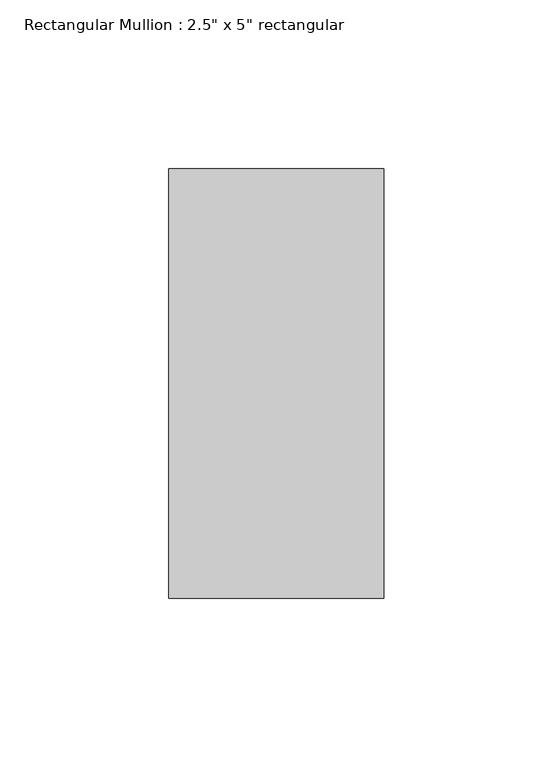
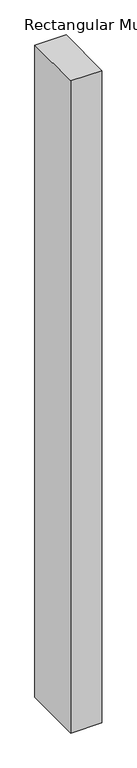
"""IFC4 building model written with IfcOpenShell, lengths in millimetres: member geometry."""

from ifc_helpers import new_model, si_unit, frame, origin, place, context, project, spatial, polyline, outline, extrude, source, transform, mapped, element, save


def member_6ba49134(model_context):
    return source(origin(), model_context, "Body", "SweptSolid", [
        extrude(outline(polyline([(31.75, 63.5), (31.75, -63.5), (-31.75, -63.5), (-31.75, 63.5), (31.75, 63.5)])), frame((0.0, 0.0, -1408.1788335), z_axis=(0.0, 0.0, 1.0), x_axis=(1.0, 0.0, 0.0)), (0.0, 0.0, 1.0), 1408.1788335),
    ])


if __name__ == "__main__":
    model = new_model("IFC4")
    model_context = context("Model", 3, world=origin())
    ifc_project = project(units=[si_unit("LENGTHUNIT", "METRE", prefix="MILLI")], contexts=[model_context])
    site = spatial("IfcSite", under=ifc_project)
    building = spatial("IfcBuilding", under=site)
    placement = place(None, origin())
    member_shape = member_6ba49134(model_context)
    element("IfcMember", 1, ObjectType="Rectangular Mullion : 2.5\" x 5\" rectangular", at=placement, inside=building, context=model_context, shape_type="MappedRepresentation", body=[
        mapped(member_shape, transform((0.0, 0.0, 0.0), x_axis=(1.0, 0.0, 0.0), y_axis=(0.0, 1.0, 0.0), z_axis=(0.0, 0.0, 1.0))),
    ])
    save(model, "model.ifc")

# Revit data of these elements
# Type "Rectangular Mullion : 2.5\" x 5\" rectangular"
#   built-in parameter 1007304 = 0.416667 (stored number, unit not read)
#   built-in parameter 1007301 = 0.104167 (stored number, unit not read)
#   built-in parameter 1007300 = 0.104167 (stored number, unit not read)
# Element 1 (IfcMember, "Rectangular Mullion : 2.5\" x 5\" rectangular")
#   Materials on its faces: "Aluminum"
# Materials
#   "Aluminum": class "Metal", colour RGB 247 247 247, transparency 0, Description = "Aluminum 6061", Cost = 0
